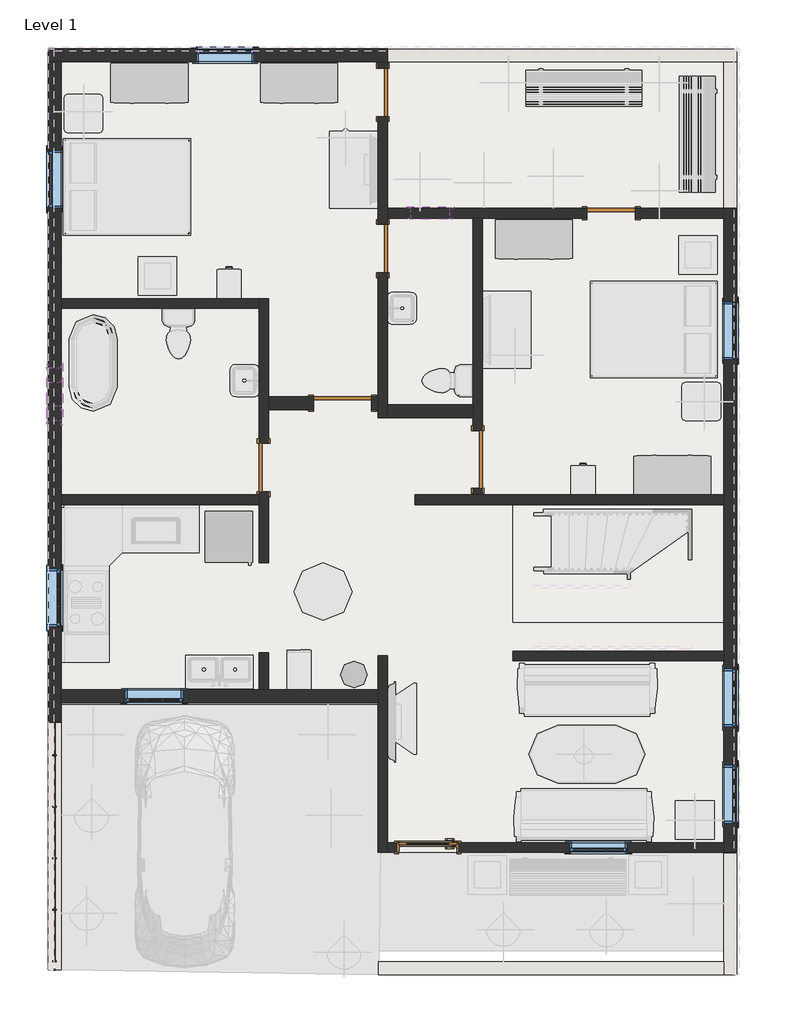
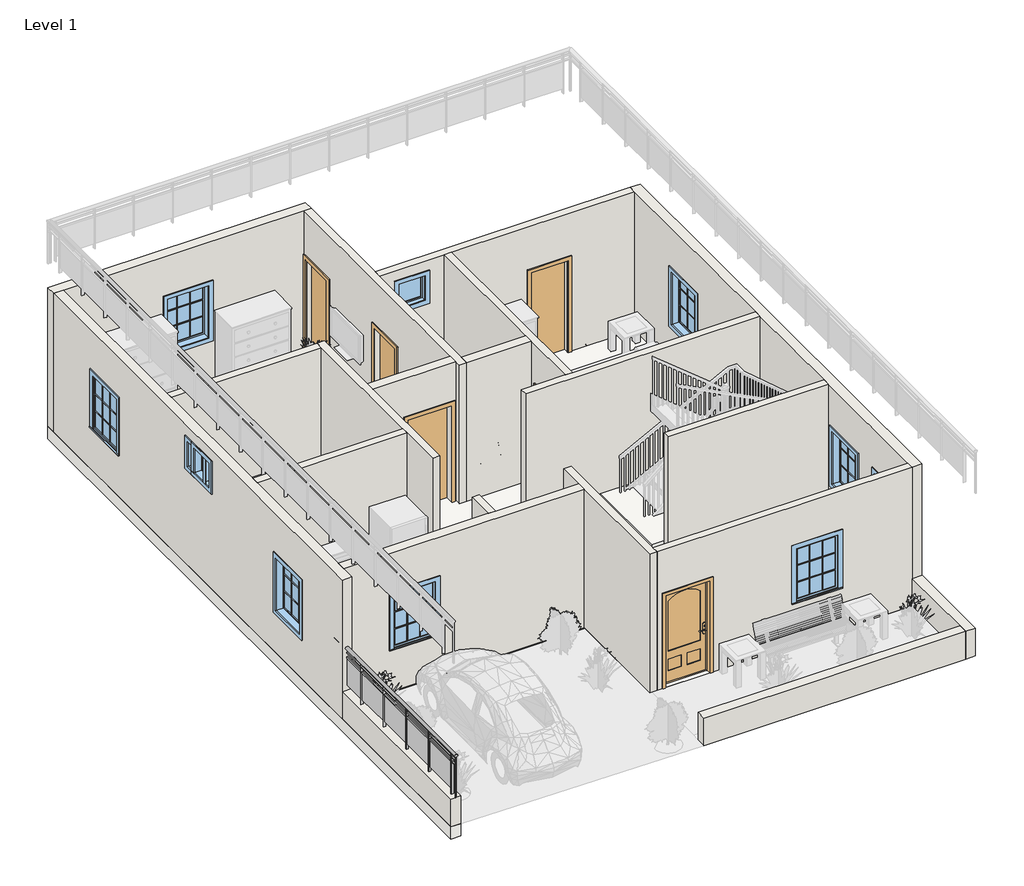
# One storey, part 1 of 4: 22 walls, 11 windows, 7 doors, 1 railing, 1 roof, 1 slab.
"""IFC4 building model written with IfcOpenShell, lengths in millimetres."""

from ifc_helpers import new_model, si_unit, point, frame, origin, origin_with_axes, place, context, project, spatial, polyline, ellipse_curve, trimmed, outline, extrude, faceted_brep, transform, mapped, element, save
from ifc_brep_helpers import plane_surface, extruded_surface, advanced_brep
from components import door_808aeb8e, door_255cab33, door_54dd4da4, door_16372e1c, window_29c06734, window_ce5e1bf6, window_5c190c7e, window_e41d21a6, window_3d781103

model = new_model("IFC4")

# Units and contexts
model_context = context("Model", 3, world=origin())
ifc_project = project(units=[si_unit("LENGTHUNIT", "METRE", prefix="MILLI")], contexts=[model_context])

# Site, building, storey
site = spatial("IfcSite", under=ifc_project)
building = spatial("IfcBuilding", under=site)
storey = spatial("IfcBuildingStorey", under=building, Name="Level 1", Elevation=0.0)

# Doors
placement = place(None, origin())
door_shape = door_808aeb8e(model_context)
element("IfcDoor", 1, ObjectType="36\" x 80\"", at=placement, inside=storey, context=model_context, shape_type="MappedRepresentation", body=[
    mapped(door_shape, transform((-6988.7866955, 3103.4537933, 0.0), x_axis=(1.0, 0.0, 0.0), y_axis=(0.0, 1.0, 0.0), z_axis=(0.0, 0.0, 1.0))),
])
door_2_shape = door_255cab33(model_context)
element("IfcDoor", 2, ObjectType="Single-Flush : 30\" x 80\"", at=placement, inside=storey, context=model_context, shape_type="MappedRepresentation", body=[
    mapped(door_2_shape, transform((-9579.5866955, 9094.6787933, 0.0), x_axis=(0.0, -1.0, 0.0), y_axis=(1.0, 0.0, 0.0), z_axis=(0.0, 0.0, 1.0))),
])
element("IfcDoor", 3, ObjectType="Single-Flush : 30\" x 80\"", at=placement, inside=storey, context=model_context, shape_type="MappedRepresentation", body=[
    mapped(door_2_shape, transform((-7699.9866955, 12549.0787933, 0.0), x_axis=(0.0, 1.0, 0.0), y_axis=(-1.0, 0.0, 0.0), z_axis=(0.0, 0.0, 1.0))),
])
element("IfcDoor", 4, ObjectType="Single-Flush : 30\" x 80\"", at=placement, inside=storey, context=model_context, shape_type="MappedRepresentation", body=[
    mapped(door_2_shape, transform((-7699.9866955, 15012.8787933, 0.0), x_axis=(0.0, 1.0, 0.0), y_axis=(-1.0, 0.0, 0.0), z_axis=(0.0, 0.0, 1.0))),
])
element("IfcDoor", 5, ObjectType="Single-Flush : 30\" x 80\"", at=placement, inside=storey, context=model_context, shape_type="MappedRepresentation", body=[
    mapped(door_2_shape, transform((-4093.1866955, 13107.8787933, 0.0), x_axis=(-1.0, 0.0, 0.0), y_axis=(0.0, -1.0, 0.0), z_axis=(0.0, 0.0, 1.0))),
])
door_3_shape = door_54dd4da4(model_context)
element("IfcDoor", 6, ObjectType="Single-Flush : 36\" x 84\"", at=placement, inside=storey, context=model_context, shape_type="MappedRepresentation", body=[
    mapped(door_3_shape, transform((-8334.9866955, 10110.6787933, 0.0), x_axis=(1.0, 0.0, 0.0), y_axis=(0.0, 1.0, 0.0), z_axis=(0.0, 0.0, 1.0))),
])
door_4_shape = door_16372e1c(model_context)
element("IfcDoor", 7, ObjectType="Single-Flush : 36\" x 84\"", at=placement, inside=storey, context=model_context, shape_type="MappedRepresentation", body=[
    mapped(door_4_shape, transform((-6201.3866955, 9221.6787933, 0.0), x_axis=(0.0, -1.0, 0.0), y_axis=(1.0, 0.0, 0.0), z_axis=(0.0, 0.0, 1.0))),
])

# Railing
element("IfcRailing", 8, ObjectType="Glass Panel - Bottom Fill", at=placement, inside=storey, context=model_context, shape_type="SolidModel", body=[
    advanced_brep(
    [(-12843.4866955, 5500.5787933, 1524.0), (-12919.6866955, 5500.5787933, 1524.0), (-12843.4866955, 1169.8787933, 1524.0), (-12919.6866955, 1169.8787933, 1524.0)],
    [
        (0, 1, ellipse_curve(frame((-12881.5866955, 5500.5787933, 1524.0), z_axis=(0.0, 1.0, 0.0), x_axis=(-1.0, 0.0, 0.0)), 38.1, 28.575)),
        (1, 0, ellipse_curve(frame((-12881.5866955, 5500.5787933, 1524.0), z_axis=(0.0, 1.0, 0.0), x_axis=(-1.0, 0.0, 0.0)), 38.1, 28.575)),
        (2, 3, ellipse_curve(frame((-12881.5866955, 1169.8787933, 1524.0), z_axis=(0.0, -1.0, 0.0), x_axis=(-1.0, 0.0, 0.0)), 38.1, 28.575)),
        (3, 2, ellipse_curve(frame((-12881.5866955, 1169.8787933, 1524.0), z_axis=(0.0, -1.0, 0.0), x_axis=(-1.0, 0.0, 0.0)), 38.1, 28.575)),
        (0, 2),
        (3, 1),
    ],
    [
        plane_surface(frame((-12881.5866955, 5500.5787933, 1524.0), z_axis=(0.0, 1.0, 0.0), x_axis=(0.0, 0.0, -1.0))),
        plane_surface(frame((-12881.5866955, 1169.8787933, 1524.0), z_axis=(0.0, -1.0, 0.0), x_axis=(0.0, 0.0, -1.0))),
        extruded_surface(trimmed(ellipse_curve(frame((-12881.5866955, 1169.8787933, 1524.0), z_axis=(0.0, 1.0, 0.0), x_axis=(-1.0, 0.0, 0.0)), 38.1, 28.575), [point((-12843.4866955, 1169.8787933, 1524.0))], [point((-12919.6866955, 1169.8787933, 1524.0))], True, "CARTESIAN"), (0.0, 4330.7, 0.0), 4330.7),
        extruded_surface(trimmed(ellipse_curve(frame((-12881.5866955, 1169.8787933, 1524.0), z_axis=(0.0, 1.0, 0.0), x_axis=(-1.0, 0.0, 0.0)), 38.1, 28.575), [point((-12919.6866955, 1169.8787933, 1524.0))], [point((-12843.4866955, 1169.8787933, 1524.0))], True, "CARTESIAN"), (0.0, 4330.7, 0.0), 4330.7),
    ],
    [
        (0, [[1, 2]]),
        (1, [[3, 4]]),
        (2, [[-1, 5, -4, 6]]),
        (3, [[-2, -6, -3, -5]]),
    ],
),
    extrude(outline(polyline([(-12894.2866955, 5500.5787933), (-12868.8866955, 5500.5787933), (-12868.8866955, 1169.8787933), (-12894.2866955, 1169.8787933), (-12894.2866955, 5500.5787933)])), frame((0.0, 0.0, 1409.7), z_axis=(0.0, 0.0, 1.0), x_axis=(1.0, 0.0, 0.0)), (0.0, 0.0, 1.0), 25.4),
    extrude(outline(polyline([(-12894.2866955, 5500.5787933), (-12868.8866955, 5500.5787933), (-12868.8866955, 1169.8787933), (-12894.2866955, 1169.8787933), (-12894.2866955, 5500.5787933)])), frame((0.0, 0.0, 1308.1), z_axis=(0.0, 0.0, 1.0), x_axis=(1.0, 0.0, 0.0)), (0.0, 0.0, 1.0), 25.4),
    extrude(outline(polyline([(-12906.9866955, 1309.5787933), (-12856.1866955, 1309.5787933), (-12856.1866955, 1296.8787933), (-12906.9866955, 1296.8787933), (-12906.9866955, 1309.5787933)])), frame((0.0, 0.0, 609.6), z_axis=(0.0, 0.0, 1.0), x_axis=(1.0, 0.0, 0.0)), (0.0, 0.0, 1.0), 885.6788223),
    extrude(outline(polyline([(-12875.0515385, 2116.0287933), (-12875.0515385, 1303.2287933), (-12881.4015385, 1303.2287933), (-12881.4015385, 2116.0287933), (-12875.0515385, 2116.0287933)])), frame((0.0, 0.0, 711.2), z_axis=(0.0, 0.0, 1.0), x_axis=(1.0, 0.0, 0.0)), (0.0, 0.0, 1.0), 596.9),
    extrude(outline(polyline([(-12906.9866955, 2122.3787933), (-12856.1866955, 2122.3787933), (-12856.1866955, 2109.6787933), (-12906.9866955, 2109.6787933), (-12906.9866955, 2122.3787933)])), frame((0.0, 0.0, 609.6), z_axis=(0.0, 0.0, 1.0), x_axis=(1.0, 0.0, 0.0)), (0.0, 0.0, 1.0), 885.6788223),
    extrude(outline(polyline([(-12875.0515385, 2928.8287933), (-12875.0515385, 2116.0287933), (-12881.4015385, 2116.0287933), (-12881.4015385, 2928.8287933), (-12875.0515385, 2928.8287933)])), frame((0.0, 0.0, 711.2), z_axis=(0.0, 0.0, 1.0), x_axis=(1.0, 0.0, 0.0)), (0.0, 0.0, 1.0), 596.9),
    extrude(outline(polyline([(-12906.9866955, 2935.1787933), (-12856.1866955, 2935.1787933), (-12856.1866955, 2922.4787933), (-12906.9866955, 2922.4787933), (-12906.9866955, 2935.1787933)])), frame((0.0, 0.0, 609.6), z_axis=(0.0, 0.0, 1.0), x_axis=(1.0, 0.0, 0.0)), (0.0, 0.0, 1.0), 885.6788223),
    extrude(outline(polyline([(-12875.0515385, 3741.6287933), (-12875.0515385, 2928.8287933), (-12881.4015385, 2928.8287933), (-12881.4015385, 3741.6287933), (-12875.0515385, 3741.6287933)])), frame((0.0, 0.0, 711.2), z_axis=(0.0, 0.0, 1.0), x_axis=(1.0, 0.0, 0.0)), (0.0, 0.0, 1.0), 596.9),
    extrude(outline(polyline([(-12906.9866955, 3747.9787933), (-12856.1866955, 3747.9787933), (-12856.1866955, 3735.2787933), (-12906.9866955, 3735.2787933), (-12906.9866955, 3747.9787933)])), frame((0.0, 0.0, 609.6), z_axis=(0.0, 0.0, 1.0), x_axis=(1.0, 0.0, 0.0)), (0.0, 0.0, 1.0), 885.6788223),
    extrude(outline(polyline([(-12875.0515385, 4554.4287933), (-12875.0515385, 3741.6287933), (-12881.4015385, 3741.6287933), (-12881.4015385, 4554.4287933), (-12875.0515385, 4554.4287933)])), frame((0.0, 0.0, 711.2), z_axis=(0.0, 0.0, 1.0), x_axis=(1.0, 0.0, 0.0)), (0.0, 0.0, 1.0), 596.9),
    extrude(outline(polyline([(-12906.9866955, 4560.7787933), (-12856.1866955, 4560.7787933), (-12856.1866955, 4548.0787933), (-12906.9866955, 4548.0787933), (-12906.9866955, 4560.7787933)])), frame((0.0, 0.0, 609.6), z_axis=(0.0, 0.0, 1.0), x_axis=(1.0, 0.0, 0.0)), (0.0, 0.0, 1.0), 885.6788223),
    extrude(outline(polyline([(-12875.0515385, 5367.2287933), (-12875.0515385, 4554.4287933), (-12881.4015385, 4554.4287933), (-12881.4015385, 5367.2287933), (-12875.0515385, 5367.2287933)])), frame((0.0, 0.0, 711.2), z_axis=(0.0, 0.0, 1.0), x_axis=(1.0, 0.0, 0.0)), (0.0, 0.0, 1.0), 596.9),
    extrude(outline(polyline([(-12906.9866955, 5373.5787933), (-12856.1866955, 5373.5787933), (-12856.1866955, 5360.8787933), (-12906.9866955, 5360.8787933), (-12906.9866955, 5373.5787933)])), frame((0.0, 0.0, 609.6), z_axis=(0.0, 0.0, 1.0), x_axis=(1.0, 0.0, 0.0)), (0.0, 0.0, 1.0), 885.6788223),
    extrude(outline(polyline([(-12891.1116955, 1182.5787933), (-12872.0616955, 1182.5787933), (-12872.0616955, 1163.5287933), (-12891.1116955, 1163.5287933), (-12891.1116955, 1182.5787933)])), frame((0.0, 0.0, 609.6), z_axis=(0.0, 0.0, 1.0), x_axis=(1.0, 0.0, 0.0)), (0.0, 0.0, 1.0), 885.6788223),
    extrude(outline(polyline([(-12891.1116955, 5506.9287933), (-12872.0616955, 5506.9287933), (-12872.0616955, 5487.8787933), (-12891.1116955, 5487.8787933), (-12891.1116955, 5506.9287933)])), frame((0.0, 0.0, 609.6), z_axis=(0.0, 0.0, 1.0), x_axis=(1.0, 0.0, 0.0)), (0.0, 0.0, 1.0), 885.6788223),
])

# Roof
element("IfcRoof", 9, ObjectType="Generic - 12\"", at=placement, inside=storey, context=model_context, shape_type="SweptSolid", body=[
    extrude(outline(polyline([(-5642.5866955, 8510.4787933), (-2111.9866955, 8510.4787933), (-2111.9866955, 6655.1793988), (-5642.5866955, 6655.1793988), (-5642.5866955, 8510.4787933)])), origin_with_axes(), (0.0, 0.0, 1.0), 304.8),
])

# Slab
element("IfcSlab", 10, ObjectType="Wood Joist 10\" - Wood Finish", at=placement, inside=storey, context=model_context, shape_type="SweptSolid", body=[
    extrude(outline(polyline([(-2111.9866955, 15698.6787933), (-2111.9866955, 3024.0787933), (-7776.1866955, 3024.0787933), (-7776.1866955, 5360.8787933), (-12754.5866955, 5360.8787933), (-12779.9866955, 5360.8787933), (-12779.9866955, 1169.8787933), (-12983.1866955, 1169.8787933), (-12983.1866955, 15698.6787933), (-2111.9866955, 15698.6787933)])), frame((0.0, 0.0, -273.05), z_axis=(0.0, 0.0, 1.0), x_axis=(1.0, 0.0, 0.0)), (0.0, 0.0, 1.0), 273.05),
])

# Walls
element("IfcWall", 11, ObjectType="Generic - 8\"", at=placement, inside=storey, context=model_context, shape_type="Brep", body=[
    faceted_brep([(-12983.1866955, 15495.4787933, 0.0), (-12779.9866955, 15495.4787933, 0.0), (-7776.1866955, 15495.4787933, 0.0), (-7699.9866955, 15495.4787933, 0.0), (-7699.9866955, 15495.4787933, 609.6), (-7623.7866955, 15495.4787933, 609.6), (-7623.7866955, 15495.4787933, 3048.0), (-7776.1866955, 15495.4787933, 3048.0), (-12779.9866955, 15495.4787933, 3048.0), (-12983.1866955, 15495.4787933, 3048.0), (-9731.9866955, 15495.4787933, 2133.6), (-9731.9866955, 15495.4787933, 914.4), (-10646.3866955, 15495.4787933, 914.4), (-10646.3866955, 15495.4787933, 2133.6), (-12983.1866955, 15698.6787933, 0.0), (-12983.1866955, 15698.6787933, 3048.0), (-7623.7866955, 15698.6787933, 3048.0), (-7623.7866955, 15698.6787933, 609.6), (-7699.9866955, 15698.6787933, 609.6), (-7699.9866955, 15698.6787933, 0.0), (-9731.9866955, 15698.6787933, 2133.6), (-10646.3866955, 15698.6787933, 2133.6), (-10646.3866955, 15698.6787933, 914.4), (-9731.9866955, 15698.6787933, 914.4)], [[[0, 1, 2, 3, 4, 5, 6, 7, 8, 9], [10, 11, 12, 13]], [[14, 15, 16, 17, 18, 19], [20, 21, 22, 23]], [[3, 2, 1, 0, 14, 19]], [[0, 9, 15, 14]], [[11, 10, 20, 23]], [[12, 11, 23, 22]], [[13, 12, 22, 21]], [[10, 13, 21, 20]], [[4, 3, 19, 18]], [[17, 5, 4, 18]], [[6, 5, 17, 16]], [[9, 8, 7, 6, 16, 15]]]),
])
element("IfcWall", 12, ObjectType="Generic - 8\"", at=placement, inside=storey, context=model_context, shape_type="Brep", body=[
    faceted_brep([(-2315.1866955, 15495.4787933, 0.0), (-2315.1866955, 13184.0787933, 0.0), (-2315.1866955, 13107.8787933, 0.0), (-2315.1866955, 13107.8787933, 609.6), (-2315.1866955, 13184.0787933, 609.6), (-2315.1866955, 15495.4787933, 609.6), (-2111.9866955, 15495.4787933, 0.0), (-2111.9866955, 15495.4787933, 609.6), (-2111.9866955, 13184.0787933, 609.6), (-2111.9866955, 13107.8787933, 609.6), (-2111.9866955, 13107.8787933, 0.0)], [[[0, 1, 2, 3, 4, 5]], [[6, 7, 8, 9, 10]], [[2, 1, 0, 6, 10]], [[3, 2, 10, 9]], [[5, 4, 3, 9, 8, 7]], [[0, 5, 7, 6]]]),
])
element("IfcWall", 13, ObjectType="Generic - 8\"", at=placement, inside=storey, context=model_context, shape_type="SweptSolid", body=[
    extrude(outline(polyline([(-7763.4866955, 1296.8787933), (-2315.1866955, 1296.8787933), (-2315.1866955, 1093.6787933), (-7763.4866955, 1093.6787933), (-7763.4866955, 1296.8787933)])), origin_with_axes(), (0.0, 0.0, 1.0), 609.6),
])
element("IfcWall", 14, ObjectType="Generic - 8\"", at=placement, inside=storey, context=model_context, shape_type="SweptSolid", body=[
    extrude(outline(polyline([(-12779.9866955, 5068.7787933), (-12779.9866955, 1169.8787933), (-12983.1866955, 1169.8787933), (-12983.1866955, 5068.7787933), (-12779.9866955, 5068.7787933)])), origin_with_axes(), (0.0, 0.0, 1.0), 609.6),
])
element("IfcWall", 15, ObjectType="Generic - 8\"", at=placement, inside=storey, context=model_context, shape_type="SweptSolid", body=[
    extrude(outline(polyline([(2133.6, -7877.7866955), (0.0, -7877.7866955), (0.0, -7776.1866955), (3048.0, -7776.1866955), (3048.0, -9503.3866955), (0.0, -9503.3866955), (0.0, -8792.1866955), (2133.6, -8792.1866955), (2133.6, -7877.7866955)])), frame((0.0, 10009.0787933, 0.0), z_axis=(0.0, 1.0, 0.0), x_axis=(0.0, 0.0, 1.0)), (0.0, 0.0, 1.0), 203.2),
])
element("IfcWall", 16, ObjectType="Generic - 8\"", at=placement, inside=storey, context=model_context, shape_type="SweptSolid", body=[
    extrude(outline(polyline([(-7623.7866955, 10085.2787933), (-6277.5866955, 10085.2787933), (-6277.5866955, 9882.0787933), (-7623.7866955, 9882.0787933), (-7623.7866955, 10085.2787933)])), origin_with_axes(), (0.0, 0.0, 1.0), 3048.0),
])
element("IfcWall", 17, ObjectType="Generic - 8\"", at=placement, inside=storey, context=model_context, shape_type="Brep", body=[
    faceted_brep([(-12779.9866955, 5386.2787933, 0.0), (-7776.1866955, 5386.2787933, 0.0), (-7776.1866955, 5386.2787933, 3048.0), (-12779.9866955, 5386.2787933, 3048.0), (-11763.9866955, 5386.2787933, 2133.6), (-10849.5866955, 5386.2787933, 2133.6), (-10849.5866955, 5386.2787933, 914.4), (-11763.9866955, 5386.2787933, 914.4), (-12779.9866955, 5589.4787933, 0.0), (-12779.9866955, 5589.4787933, 3048.0), (-9655.7866955, 5589.4787933, 3048.0), (-9503.3866955, 5589.4787933, 3048.0), (-7776.1866955, 5589.4787933, 3048.0), (-7776.1866955, 5589.4787933, 0.0), (-9503.3866955, 5589.4787933, 0.0), (-9655.7866955, 5589.4787933, 0.0), (-11763.9866955, 5589.4787933, 2133.6), (-11763.9866955, 5589.4787933, 914.4), (-10849.5866955, 5589.4787933, 914.4), (-10849.5866955, 5589.4787933, 2133.6)], [[[0, 1, 2, 3], [4, 5, 6, 7]], [[8, 9, 10, 11, 12, 13, 14, 15], [16, 17, 18, 19]], [[1, 0, 8, 15, 14, 13]], [[0, 3, 9, 8]], [[2, 1, 13, 12]], [[17, 16, 4, 7]], [[18, 17, 7, 6]], [[19, 18, 6, 5]], [[16, 19, 5, 4]], [[3, 2, 12, 11, 10, 9]]]),
])
element("IfcWall", 18, ObjectType="Generic - 8\"", at=placement, inside=storey, context=model_context, shape_type="Brep", body=[
    faceted_brep([(-2315.1866955, 3011.3787933, 0.0), (-2315.1866955, 1296.8787933, 0.0), (-2315.1866955, 1093.6787933, 0.0), (-2315.1866955, 1093.6787933, 609.6), (-2315.1866955, 1296.8787933, 609.6), (-2315.1866955, 3011.3787933, 609.6), (-2111.9866955, 3011.3787933, 0.0), (-2111.9866955, 3011.3787933, 609.6), (-2111.9866955, 1093.6787933, 609.6), (-2111.9866955, 1093.6787933, 0.0)], [[[0, 1, 2, 3, 4, 5]], [[6, 7, 8, 9]], [[2, 1, 0, 6, 9]], [[5, 4, 3, 8, 7]], [[0, 5, 7, 6]], [[3, 2, 9, 8]]]),
])
element("IfcWall", 19, ObjectType="Generic - 8\"", at=placement, inside=storey, context=model_context, shape_type="Brep", body=[
    faceted_brep([(-12779.9866955, 5094.1787933, 0.0), (-12779.9866955, 5386.2787933, 0.0), (-12779.9866955, 5589.4787933, 0.0), (-12779.9866955, 8510.4787933, 0.0), (-12779.9866955, 8662.8787933, 0.0), (-12779.9866955, 11609.2787933, 0.0), (-12779.9866955, 11761.6787933, 0.0), (-12779.9866955, 15495.4787933, 0.0), (-12779.9866955, 15495.4787933, 3048.0), (-12779.9866955, 11761.6787933, 3048.0), (-12779.9866955, 11609.2787933, 3048.0), (-12779.9866955, 8662.8787933, 3048.0), (-12779.9866955, 8510.4787933, 3048.0), (-12779.9866955, 5589.4787933, 3048.0), (-12779.9866955, 5386.2787933, 3048.0), (-12779.9866955, 5094.1787933, 3048.0), (-12779.9866955, 14098.4787933, 2133.6), (-12779.9866955, 14098.4787933, 914.4), (-12779.9866955, 13184.0787933, 914.4), (-12779.9866955, 13184.0787933, 2133.6), (-12779.9866955, 7494.4787933, 2133.6), (-12779.9866955, 7494.4787933, 914.4), (-12779.9866955, 6580.0787933, 914.4), (-12779.9866955, 6580.0787933, 2133.6), (-12779.9866955, 10669.4787933, 2159.0), (-12779.9866955, 9831.2787933, 2159.0), (-12779.9866955, 9831.2787933, 2768.6), (-12779.9866955, 10669.4787933, 2768.6), (-12983.1866955, 15495.4787933, 0.0), (-12983.1866955, 5094.1787933, 0.0), (-12983.1866955, 5094.1787933, 3048.0), (-12983.1866955, 15495.4787933, 3048.0), (-12983.1866955, 14098.4787933, 2133.6), (-12983.1866955, 13184.0787933, 2133.6), (-12983.1866955, 13184.0787933, 914.4), (-12983.1866955, 14098.4787933, 914.4), (-12983.1866955, 7494.4787933, 2133.6), (-12983.1866955, 6580.0787933, 2133.6), (-12983.1866955, 6580.0787933, 914.4), (-12983.1866955, 7494.4787933, 914.4), (-12983.1866955, 10669.4787933, 2768.6), (-12983.1866955, 9831.2787933, 2768.6), (-12983.1866955, 9831.2787933, 2159.0), (-12983.1866955, 10669.4787933, 2159.0)], [[[0, 1, 2, 3, 4, 5, 6, 7, 8, 9, 10, 11, 12, 13, 14, 15], [16, 17, 18, 19], [20, 21, 22, 23], [24, 25, 26, 27]], [[28, 29, 30, 31], [32, 33, 34, 35], [36, 37, 38, 39], [40, 41, 42, 43]], [[7, 6, 5, 4, 3, 2, 1, 0, 29, 28]], [[0, 15, 30, 29]], [[8, 7, 28, 31]], [[17, 16, 32, 35]], [[18, 17, 35, 34]], [[19, 18, 34, 33]], [[16, 19, 33, 32]], [[21, 20, 36, 39]], [[22, 21, 39, 38]], [[23, 22, 38, 37]], [[20, 23, 37, 36]], [[42, 41, 26, 25]], [[42, 25, 24, 43]], [[26, 41, 40, 27]], [[43, 24, 27, 40]], [[15, 14, 13, 12, 11, 10, 9, 8, 31, 30]]]),
])
element("IfcWall", 20, ObjectType="Generic - 8\"", at=placement, inside=storey, context=model_context, shape_type="Brep", body=[
    faceted_brep([(-7699.9866955, 15495.4787933, 0.0), (-7623.7866955, 15495.4787933, 0.0), (-2315.1866955, 15495.4787933, 0.0), (-2111.9866955, 15495.4787933, 0.0), (-2111.9866955, 15495.4787933, 609.6), (-2315.1866955, 15495.4787933, 609.6), (-7623.7866955, 15495.4787933, 609.6), (-7699.9866955, 15495.4787933, 609.6), (-7699.9866955, 15698.6787933, 0.0), (-7699.9866955, 15698.6787933, 609.6), (-7623.7866955, 15698.6787933, 609.6), (-2111.9866955, 15698.6787933, 609.6), (-2111.9866955, 15698.6787933, 0.0)], [[[0, 1, 2, 3, 4, 5, 6, 7]], [[8, 9, 10, 11, 12]], [[3, 2, 1, 0, 8, 12]], [[7, 6, 5, 4, 11, 10, 9]], [[0, 7, 9, 8]], [[4, 3, 12, 11]]]),
])
element("IfcWall", 21, ObjectType="Generic - 8\"", at=placement, inside=storey, context=model_context, shape_type="Brep", body=[
    faceted_brep([(-2315.1866955, 13107.8787933, 0.0), (-2315.1866955, 13031.6787933, 0.0), (-2315.1866955, 8662.8787933, 0.0), (-2315.1866955, 8510.4787933, 0.0), (-2315.1866955, 6199.0787933, 0.0), (-2315.1866955, 6046.6787933, 0.0), (-2315.1866955, 3176.4787933, 0.0), (-2315.1866955, 3036.7787933, 0.0), (-2315.1866955, 3036.7787933, 3048.0), (-2315.1866955, 3176.4787933, 3048.0), (-2315.1866955, 6046.6787933, 3048.0), (-2315.1866955, 6199.0787933, 3048.0), (-2315.1866955, 8510.4787933, 3048.0), (-2315.1866955, 8662.8787933, 3048.0), (-2315.1866955, 13031.6787933, 3048.0), (-2315.1866955, 13184.0787933, 3048.0), (-2315.1866955, 13184.0787933, 609.6), (-2315.1866955, 13107.8787933, 609.6), (-2315.1866955, 10796.4787933, 2133.6), (-2315.1866955, 10796.4787933, 914.4), (-2315.1866955, 11710.8787933, 914.4), (-2315.1866955, 11710.8787933, 2133.6), (-2315.1866955, 3481.2787933, 2133.6), (-2315.1866955, 3481.2787933, 914.4), (-2315.1866955, 4395.6787933, 914.4), (-2315.1866955, 4395.6787933, 2133.6), (-2315.1866955, 5005.2787933, 2133.6), (-2315.1866955, 5005.2787933, 914.4), (-2315.1866955, 5919.6787933, 914.4), (-2315.1866955, 5919.6787933, 2133.6), (-2111.9866955, 13107.8787933, 0.0), (-2111.9866955, 13107.8787933, 609.6), (-2111.9866955, 13184.0787933, 609.6), (-2111.9866955, 13184.0787933, 3048.0), (-2111.9866955, 3036.7787933, 3048.0), (-2111.9866955, 3036.7787933, 0.0), (-2111.9866955, 10796.4787933, 2133.6), (-2111.9866955, 11710.8787933, 2133.6), (-2111.9866955, 11710.8787933, 914.4), (-2111.9866955, 10796.4787933, 914.4), (-2111.9866955, 3481.2787933, 2133.6), (-2111.9866955, 4395.6787933, 2133.6), (-2111.9866955, 4395.6787933, 914.4), (-2111.9866955, 3481.2787933, 914.4), (-2111.9866955, 5005.2787933, 2133.6), (-2111.9866955, 5919.6787933, 2133.6), (-2111.9866955, 5919.6787933, 914.4), (-2111.9866955, 5005.2787933, 914.4)], [[[0, 1, 2, 3, 4, 5, 6, 7, 8, 9, 10, 11, 12, 13, 14, 15, 16, 17], [18, 19, 20, 21], [22, 23, 24, 25], [26, 27, 28, 29]], [[30, 31, 32, 33, 34, 35], [36, 37, 38, 39], [40, 41, 42, 43], [44, 45, 46, 47]], [[7, 6, 5, 4, 3, 2, 1, 0, 30, 35]], [[8, 7, 35, 34]], [[18, 21, 37, 36]], [[21, 20, 38, 37]], [[20, 19, 39, 38]], [[19, 18, 36, 39]], [[22, 25, 41, 40]], [[25, 24, 42, 41]], [[24, 23, 43, 42]], [[23, 22, 40, 43]], [[26, 29, 45, 44]], [[29, 28, 46, 45]], [[28, 27, 47, 46]], [[27, 26, 44, 47]], [[0, 17, 31, 30]], [[16, 32, 31, 17]], [[16, 15, 33, 32]], [[15, 14, 13, 12, 11, 10, 9, 8, 34, 33]]]),
])
element("IfcWall", 22, ObjectType="INNER 6\"", at=placement, inside=storey, context=model_context, shape_type="Brep", body=[
    faceted_brep([(-7776.1866955, 15495.4787933, 0.0), (-7776.1866955, 15393.8787933, 0.0), (-7776.1866955, 15393.8787933, 2032.0), (-7776.1866955, 14631.8787933, 2032.0), (-7776.1866955, 14631.8787933, 0.0), (-7776.1866955, 12930.0787933, 0.0), (-7776.1866955, 12930.0787933, 2032.0), (-7776.1866955, 12168.0787933, 2032.0), (-7776.1866955, 12168.0787933, 0.0), (-7776.1866955, 10212.2787933, 0.0), (-7776.1866955, 10009.0787933, 0.0), (-7776.1866955, 9882.0787933, 0.0), (-7776.1866955, 9882.0787933, 3048.0), (-7776.1866955, 10009.0787933, 3048.0), (-7776.1866955, 10212.2787933, 3048.0), (-7776.1866955, 15495.4787933, 3048.0), (-7623.7866955, 15393.8787933, 2032.0), (-7623.7866955, 15393.8787933, 0.0), (-7623.7866955, 15495.4787933, 0.0), (-7623.7866955, 15495.4787933, 609.6), (-7623.7866955, 15495.4787933, 3048.0), (-7623.7866955, 13184.0787933, 3048.0), (-7623.7866955, 13031.6787933, 3048.0), (-7623.7866955, 10085.2787933, 3048.0), (-7623.7866955, 9882.0787933, 3048.0), (-7623.7866955, 9882.0787933, 0.0), (-7623.7866955, 10085.2787933, 0.0), (-7623.7866955, 12168.0787933, 0.0), (-7623.7866955, 12168.0787933, 2032.0), (-7623.7866955, 12930.0787933, 2032.0), (-7623.7866955, 12930.0787933, 0.0), (-7623.7866955, 13031.6787933, 0.0), (-7623.7866955, 13184.0787933, 0.0), (-7623.7866955, 14631.8787933, 0.0), (-7623.7866955, 14631.8787933, 2032.0), (-7699.9866955, 15495.4787933, 0.0)], [[[0, 1, 2, 3, 4, 5, 6, 7, 8, 9, 10, 11, 12, 13, 14, 15]], [[16, 17, 18, 19, 20, 21, 22, 23, 24, 25, 26, 27, 28, 29, 30, 31, 32, 33, 34]], [[27, 26, 25, 11, 10, 9, 8]], [[18, 17, 1, 0, 35]], [[33, 32, 31, 30, 5, 4]], [[12, 11, 25, 24]], [[6, 5, 30, 29]], [[7, 6, 29, 28]], [[8, 7, 28, 27]], [[2, 1, 17, 16]], [[3, 2, 16, 34]], [[4, 3, 34, 33]], [[15, 20, 19, 18, 35, 0]], [[15, 14, 13, 12, 24, 23, 22, 21, 20]]]),
])
element("IfcWall", 23, ObjectType="INNER 6\"", at=placement, inside=storey, context=model_context, shape_type="SweptSolid", body=[
    extrude(outline(polyline([(-9503.3866955, 6173.6787933), (-9503.3866955, 5589.4787933), (-9655.7866955, 5589.4787933), (-9655.7866955, 6173.6787933), (-9503.3866955, 6173.6787933)])), origin_with_axes(), (0.0, 0.0, 1.0), 3048.0),
])
element("IfcWall", 24, ObjectType="INNER 6\"", at=placement, inside=storey, context=model_context, shape_type="SweptSolid", body=[
    extrude(outline(polyline([(-12779.9866955, 11761.6787933), (-9655.7866955, 11761.6787933), (-9655.7866955, 11609.2787933), (-12779.9866955, 11609.2787933), (-12779.9866955, 11761.6787933)])), origin_with_axes(), (0.0, 0.0, 1.0), 3048.0),
])
element("IfcWall", 25, ObjectType="INNER 6\"", at=placement, inside=storey, context=model_context, shape_type="SweptSolid", body=[
    extrude(outline(polyline([(-9655.7866955, 8510.4787933), (-12779.9866955, 8510.4787933), (-12779.9866955, 8662.8787933), (-9655.7866955, 8662.8787933), (-9655.7866955, 8510.4787933)])), origin_with_axes(), (0.0, 0.0, 1.0), 3048.0),
])
element("IfcWall", 26, ObjectType="INNER 6\"", at=placement, inside=storey, context=model_context, shape_type="Brep", body=[
    faceted_brep([(-7191.9866955, 8510.4787933, 0.0), (-2315.1866955, 8510.4787933, 0.0), (-2315.1866955, 8510.4787933, 3048.0), (-7191.9866955, 8510.4787933, 3048.0), (-7191.9866955, 8662.8787933, 0.0), (-7191.9866955, 8662.8787933, 3048.0), (-6277.5866955, 8662.8787933, 3048.0), (-6125.1866955, 8662.8787933, 3048.0), (-2315.1866955, 8662.8787933, 3048.0), (-2315.1866955, 8662.8787933, 0.0), (-6125.1866955, 8662.8787933, 0.0), (-6277.5866955, 8662.8787933, 0.0)], [[[0, 1, 2, 3]], [[4, 5, 6, 7, 8, 9, 10, 11]], [[1, 0, 4, 11, 10, 9]], [[0, 3, 5, 4]], [[2, 1, 9, 8]], [[3, 2, 8, 7, 6, 5]]]),
])
element("IfcWall", 27, ObjectType="INNER 6\"", at=placement, inside=storey, context=model_context, shape_type="Brep", body=[
    faceted_brep([(-7623.7866955, 13031.6787933, 0.0), (-6277.5866955, 13031.6787933, 0.0), (-6125.1866955, 13031.6787933, 0.0), (-4474.1866955, 13031.6787933, 0.0), (-4474.1866955, 13031.6787933, 2032.0), (-3712.1866955, 13031.6787933, 2032.0), (-3712.1866955, 13031.6787933, 0.0), (-2315.1866955, 13031.6787933, 0.0), (-2315.1866955, 13031.6787933, 3048.0), (-6125.1866955, 13031.6787933, 3048.0), (-6277.5866955, 13031.6787933, 3048.0), (-7623.7866955, 13031.6787933, 3048.0), (-6645.8866955, 13031.6787933, 2768.6), (-6645.8866955, 13031.6787933, 2159.0), (-7255.4866955, 13031.6787933, 2159.0), (-7255.4866955, 13031.6787933, 2768.6), (-4474.1866955, 13184.0787933, 2032.0), (-4474.1866955, 13184.0787933, 0.0), (-7623.7866955, 13184.0787933, 0.0), (-7623.7866955, 13184.0787933, 3048.0), (-2315.1866955, 13184.0787933, 3048.0), (-2315.1866955, 13184.0787933, 609.6), (-2315.1866955, 13184.0787933, 0.0), (-3712.1866955, 13184.0787933, 0.0), (-3712.1866955, 13184.0787933, 2032.0), (-6645.8866955, 13184.0787933, 2768.6), (-7255.4866955, 13184.0787933, 2768.6), (-7255.4866955, 13184.0787933, 2159.0), (-6645.8866955, 13184.0787933, 2159.0), (-2315.1866955, 13107.8787933, 0.0)], [[[0, 1, 2, 3, 4, 5, 6, 7, 8, 9, 10, 11], [12, 13, 14, 15]], [[16, 17, 18, 19, 20, 21, 22, 23, 24], [25, 26, 27, 28]], [[23, 22, 29, 7, 6]], [[18, 17, 3, 2, 1, 0]], [[0, 11, 19, 18]], [[4, 3, 17, 16]], [[5, 4, 16, 24]], [[6, 5, 24, 23]], [[13, 12, 25, 28]], [[14, 13, 28, 27]], [[15, 14, 27, 26]], [[12, 15, 26, 25]], [[7, 29, 22, 21, 20, 8]], [[11, 10, 9, 8, 20, 19]]]),
])
element("IfcWall", 28, ObjectType="INNER 6\"", at=placement, inside=storey, context=model_context, shape_type="Brep", body=[
    faceted_brep([(-6277.5866955, 8764.4787933, 2133.6), (-6277.5866955, 8764.4787933, 0.0), (-6277.5866955, 8662.8787933, 0.0), (-6277.5866955, 8662.8787933, 3048.0), (-6277.5866955, 9882.0787933, 3048.0), (-6277.5866955, 10085.2787933, 3048.0), (-6277.5866955, 13031.6787933, 3048.0), (-6277.5866955, 13031.6787933, 0.0), (-6277.5866955, 10085.2787933, 0.0), (-6277.5866955, 9882.0787933, 0.0), (-6277.5866955, 9678.8787933, 0.0), (-6277.5866955, 9678.8787933, 2133.6), (-6125.1866955, 8662.8787933, 0.0), (-6125.1866955, 8764.4787933, 0.0), (-6125.1866955, 8764.4787933, 2133.6), (-6125.1866955, 9678.8787933, 2133.6), (-6125.1866955, 9678.8787933, 0.0), (-6125.1866955, 13031.6787933, 0.0), (-6125.1866955, 13031.6787933, 3048.0), (-6125.1866955, 8662.8787933, 3048.0)], [[[0, 1, 2, 3, 4, 5, 6, 7, 8, 9, 10, 11]], [[12, 13, 14, 15, 16, 17, 18, 19]], [[2, 1, 13, 12]], [[10, 9, 8, 7, 17, 16]], [[7, 6, 18, 17]], [[3, 2, 12, 19]], [[14, 13, 1, 0]], [[15, 14, 0, 11]], [[16, 15, 11, 10]], [[6, 5, 4, 3, 19, 18]]]),
])
element("IfcWall", 29, ObjectType="INNER 6\"", at=placement, inside=storey, context=model_context, shape_type="Brep", body=[
    faceted_brep([(-7623.7866955, 3024.0787933, 0.0), (-7623.7866955, 3176.4787933, 0.0), (-7623.7866955, 6122.8787933, 0.0), (-7623.7866955, 6122.8787933, 3048.0), (-7623.7866955, 3176.4787933, 3048.0), (-7623.7866955, 3024.0787933, 3048.0), (-7776.1866955, 3024.0787933, 0.0), (-7776.1866955, 3024.0787933, 3048.0), (-7776.1866955, 5386.2787933, 3048.0), (-7776.1866955, 5589.4787933, 3048.0), (-7776.1866955, 6122.8787933, 3048.0), (-7776.1866955, 6122.8787933, 0.0), (-7776.1866955, 5589.4787933, 0.0), (-7776.1866955, 5386.2787933, 0.0)], [[[0, 1, 2, 3, 4, 5]], [[6, 7, 8, 9, 10, 11, 12, 13]], [[2, 1, 0, 6, 13, 12, 11]], [[3, 2, 11, 10]], [[0, 5, 7, 6]], [[5, 4, 3, 10, 9, 8, 7]]]),
])
element("IfcWall", 30, ObjectType="INNER 6\"", at=placement, inside=storey, context=model_context, shape_type="Brep", body=[
    faceted_brep([(-7623.7866955, 3176.4787933, 0.0), (-7623.7866955, 3176.4787933, 3048.0), (-2315.1866955, 3176.4787933, 3048.0), (-2315.1866955, 3176.4787933, 0.0), (-6506.1866955, 3176.4787933, 0.0), (-6506.1866955, 3176.4787933, 2057.4), (-7471.3866955, 3176.4787933, 2057.4), (-7471.3866955, 3176.4787933, 0.0), (-4753.5866955, 3176.4787933, 2133.6), (-4753.5866955, 3176.4787933, 914.4), (-3839.1866955, 3176.4787933, 914.4), (-3839.1866955, 3176.4787933, 2133.6), (-7623.7866955, 3024.0787933, 3048.0), (-7623.7866955, 3024.0787933, 0.0), (-7471.3866955, 3024.0787933, 0.0), (-7471.3866955, 3024.0787933, 2057.4), (-6506.1866955, 3024.0787933, 2057.4), (-6506.1866955, 3024.0787933, 0.0), (-2315.1866955, 3024.0787933, 0.0), (-2315.1866955, 3024.0787933, 3048.0), (-4753.5866955, 3024.0787933, 2133.6), (-3839.1866955, 3024.0787933, 2133.6), (-3839.1866955, 3024.0787933, 914.4), (-4753.5866955, 3024.0787933, 914.4), (-2315.1866955, 3036.7787933, 0.0), (-2315.1866955, 3036.7787933, 3048.0)], [[[0, 1, 2, 3, 4, 5, 6, 7], [8, 9, 10, 11]], [[12, 13, 14, 15, 16, 17, 18, 19], [20, 21, 22, 23]], [[13, 0, 7, 14]], [[3, 24, 18, 17, 4]], [[1, 0, 13, 12]], [[16, 5, 4, 17]], [[5, 16, 15, 6]], [[6, 15, 14, 7]], [[3, 2, 25, 19, 18, 24]], [[9, 8, 20, 23]], [[10, 9, 23, 22]], [[11, 10, 22, 21]], [[8, 11, 21, 20]], [[2, 1, 12, 19, 25]]]),
])
element("IfcWall", 31, ObjectType="INNER 6\"", at=placement, inside=storey, context=model_context, shape_type="Brep", body=[
    faceted_brep([(-9503.3866955, 7596.0787933, 0.0), (-9503.3866955, 8713.6787933, 0.0), (-9503.3866955, 8713.6787933, 2032.0), (-9503.3866955, 9475.6787933, 2032.0), (-9503.3866955, 9475.6787933, 0.0), (-9503.3866955, 10009.0787933, 0.0), (-9503.3866955, 10212.2787933, 0.0), (-9503.3866955, 11761.6787933, 0.0), (-9503.3866955, 11761.6787933, 3048.0), (-9503.3866955, 10212.2787933, 3048.0), (-9503.3866955, 10009.0787933, 3048.0), (-9503.3866955, 7596.0787933, 3048.0), (-9655.7866955, 8713.6787933, 2032.0), (-9655.7866955, 8713.6787933, 0.0), (-9655.7866955, 8662.8787933, 0.0), (-9655.7866955, 8510.4787933, 0.0), (-9655.7866955, 7596.0787933, 0.0), (-9655.7866955, 7596.0787933, 3048.0), (-9655.7866955, 8510.4787933, 3048.0), (-9655.7866955, 8662.8787933, 3048.0), (-9655.7866955, 11609.2787933, 3048.0), (-9655.7866955, 11761.6787933, 3048.0), (-9655.7866955, 11761.6787933, 0.0), (-9655.7866955, 11609.2787933, 0.0), (-9655.7866955, 9475.6787933, 0.0), (-9655.7866955, 9475.6787933, 2032.0)], [[[0, 1, 2, 3, 4, 5, 6, 7, 8, 9, 10, 11]], [[12, 13, 14, 15, 16, 17, 18, 19, 20, 21, 22, 23, 24, 25]], [[24, 23, 22, 7, 6, 5, 4]], [[16, 15, 14, 13, 1, 0]], [[0, 11, 17, 16]], [[8, 7, 22, 21]], [[4, 3, 25, 24]], [[3, 2, 12, 25]], [[2, 1, 13, 12]], [[11, 10, 9, 8, 21, 20, 19, 18, 17]]]),
])
element("IfcWall", 32, ObjectType="INNER 6\"", at=placement, inside=storey, context=model_context, shape_type="SweptSolid", body=[
    extrude(outline(polyline([(-5642.5866955, 6199.0787933), (-2315.1866955, 6199.0787933), (-2315.1866955, 6046.6787933), (-5642.5866955, 6046.6787933), (-5642.5866955, 6199.0787933)])), origin_with_axes(), (0.0, 0.0, 1.0), 3048.0),
])

# Windows
window_shape = window_29c06734(model_context)
element("IfcWindow", 33, ObjectType="Casement 3x3 with Trim : 36\" x 48\"", at=placement, inside=storey, context=model_context, shape_type="MappedRepresentation", body=[
    mapped(window_shape, transform((-12881.5866955, 13641.2787933, 0.0), x_axis=(0.0, 1.0, 0.0), y_axis=(-1.0, 0.0, 0.0), z_axis=(0.0, 0.0, 1.0))),
])
element("IfcWindow", 34, ObjectType="Casement 3x3 with Trim : 36\" x 48\"", at=placement, inside=storey, context=model_context, shape_type="MappedRepresentation", body=[
    mapped(window_shape, transform((-10189.1866955, 15597.0787933, 0.0), x_axis=(1.0, 0.0, 0.0), y_axis=(0.0, 1.0, 0.0), z_axis=(0.0, 0.0, 1.0))),
])
element("IfcWindow", 35, ObjectType="Casement 3x3 with Trim : 36\" x 48\"", at=placement, inside=storey, context=model_context, shape_type="MappedRepresentation", body=[
    mapped(window_shape, transform((-2213.5866955, 11253.6787933, 0.0), x_axis=(0.0, -1.0, 0.0), y_axis=(1.0, 0.0, 0.0), z_axis=(0.0, 0.0, 1.0))),
])
element("IfcWindow", 36, ObjectType="Casement 3x3 with Trim : 36\" x 48\"", at=placement, inside=storey, context=model_context, shape_type="MappedRepresentation", body=[
    mapped(window_shape, transform((-11306.7866955, 5487.8787933, 0.0), x_axis=(-1.0, 0.0, 0.0), y_axis=(0.0, -1.0, 0.0), z_axis=(0.0, 0.0, 1.0))),
])
element("IfcWindow", 37, ObjectType="Casement 3x3 with Trim : 36\" x 48\"", at=placement, inside=storey, context=model_context, shape_type="MappedRepresentation", body=[
    mapped(window_shape, transform((-2213.5866955, 3938.4787933, 0.0), x_axis=(0.0, -1.0, 0.0), y_axis=(1.0, 0.0, 0.0), z_axis=(0.0, 0.0, 1.0))),
])
element("IfcWindow", 38, ObjectType="Casement 3x3 with Trim : 36\" x 48\"", at=placement, inside=storey, context=model_context, shape_type="MappedRepresentation", body=[
    mapped(window_shape, transform((-2213.5866955, 5462.4787933, 0.0), x_axis=(0.0, -1.0, 0.0), y_axis=(1.0, 0.0, 0.0), z_axis=(0.0, 0.0, 1.0))),
])
window_2_shape = window_ce5e1bf6(model_context)
element("IfcWindow", 39, ObjectType="Casement 3x3 with Trim : 36\" x 48\"", at=placement, inside=storey, context=model_context, shape_type="MappedRepresentation", body=[
    mapped(window_2_shape, transform((-12881.5866955, 7037.2787933, 0.0), x_axis=(0.0, 1.0, 0.0), y_axis=(-1.0, 0.0, 0.0), z_axis=(0.0, 0.0, 1.0))),
])
window_3_shape = window_5c190c7e(model_context)
element("IfcWindow", 40, ObjectType="Casement 3x3 with Trim : 36\" x 48\"", at=placement, inside=storey, context=model_context, shape_type="MappedRepresentation", body=[
    mapped(window_3_shape, transform((-4296.3866955, 3100.2787933, 0.0), x_axis=(-1.0, 0.0, 0.0), y_axis=(0.0, -1.0, 0.0), z_axis=(0.0, 0.0, 1.0))),
])
window_4_shape = window_e41d21a6(model_context)
element("IfcWindow", 41, ObjectType="Transom with Trim : 24\" x 24\"", at=placement, inside=storey, context=model_context, shape_type="MappedRepresentation", body=[
    mapped(window_4_shape, transform((-12881.5866955, 10097.9787933, 0.0), x_axis=(0.0, -1.0, 0.0), y_axis=(1.0, 0.0, 0.0), z_axis=(0.0, 0.0, 1.0))),
])
element("IfcWindow", 42, ObjectType="Transom with Trim : 24\" x 24\"", at=placement, inside=storey, context=model_context, shape_type="MappedRepresentation", body=[
    mapped(window_4_shape, transform((-12881.5866955, 10326.5787933, 0.0), x_axis=(0.0, -1.0, 0.0), y_axis=(1.0, 0.0, 0.0), z_axis=(0.0, 0.0, 1.0))),
])
window_5_shape = window_3d781103(model_context)
element("IfcWindow", 43, ObjectType="Transom with Trim : 24\" x 24\"", at=placement, inside=storey, context=model_context, shape_type="MappedRepresentation", body=[
    mapped(window_5_shape, transform((-6912.5866955, 13107.8787933, 0.0), x_axis=(1.0, 0.0, 0.0), y_axis=(0.0, 1.0, 0.0), z_axis=(0.0, 0.0, 1.0))),
])

save(model, "model.ifc")

# Revit data of these elements
# Type "36\" x 80\""
#   Type Mark = "8"
#   Assembly Code = "B2030100"
#   Analytic Construction = "French door, wood frame with single glass"
#   Threshold Offset [instance default] = 0' - 0 1/2"
#   Thickness = 0' - 1 3/8"
#   Thermal Resistance (R) = 1.0696 (h·ft²·°F)/BTU
#   Swing Angle [instance default] = 90.00°
#   Stiles = 0' - 4 3/4"
#   Rough Width = 3' - 2"
#   Rough Height = 6' - 9"
#   Radius = 1' - 8.05625"
#   Lock Rail = 0' - 7 1/8"
#   Height = 6' - 8"
#   Width = 3' - 0"
#   Heat Transfer Coefficient (U) = 0.9350 BTU/(h·ft²·°F)
#   Door Offset [instance default] = 0' - 0"
#   Bottom Rail = 0' - 9 1/2"
#   Threshold [instance default] = yes
#   Function = 1
#   Exterior Trim [instance default] = yes
#   Trim Material = Cherry
#   Threshold Material = Cherry
#   Panel Material = Cherry
#   Glazing = Glass
#   Frame Material = Cherry
#   Door Handle Material = Aluminum
#   Visual Light Transmittance = 0
#   Solar Heat Gain Coefficient = 0
#   Wall Closure = (empty or 0)
#   Construction Type = (empty or 0)
# Type "Single-Flush : 30\" x 80\""
#   Type Mark = "5"
#   Construction Type Id = "MDOOR"
#   Assembly Code = "C1020"
#   Analytic Construction = "Metal"
#   Thickness = 0' - 2"
#   Heat Transfer Coefficient (U) = 0.651978 BTU/(h·ft²·°F)
#   Height = 6' - 8"
#   Trim Projection Ext = 0' - 1"
#   Trim Projection Int = 0' - 1"
#   Trim Width = 0' - 3"
#   Width = 2' - 6"
#   Define Thermal Properties by = 1
#   Door Material = Door - Panel
#   Frame Material = Door - Frame
#   Visual Light Transmittance = 0
#   Solar Heat Gain Coefficient = 0
#   Function = (empty or 0)
#   Wall Closure = (empty or 0)
# Type "Single-Flush : 36\" x 84\""
#   Type Mark = "1"
#   Construction Type Id = "MDOOR"
#   Assembly Code = "C1020"
#   Analytic Construction = "Metal"
#   Thickness = 0' - 2"
#   Heat Transfer Coefficient (U) = 0.651978 BTU/(h·ft²·°F)
#   Height = 7' - 0"
#   Trim Projection Ext = 0' - 1"
#   Trim Projection Int = 0' - 1"
#   Trim Width = 0' - 3"
#   Width = 3' - 0"
#   Define Thermal Properties by = 1
#   Door Material = Door - Panel
#   Frame Material = Door - Frame
#   Visual Light Transmittance = 0
#   Solar Heat Gain Coefficient = 0
#   Function = (empty or 0)
#   Wall Closure = (empty or 0)
# Type "Glass Panel - Bottom Fill"
#   Assembly Code = "C2010400"
#   built-in parameter 1008612 = 0.0416667 (stored number, unit not read)
#   built-in parameter 1008611 = 0.0416667 (stored number, unit not read)
#   built-in parameter 1008609 = 0.333333 (stored number, unit not read)
#   built-in parameter 1008604 = 0.166667 (stored number, unit not read)
#   built-in parameter 1008603 = 0.166667 (stored number, unit not read)
#   Railing Height = 3' - 0"
#   built-in parameter 1008630 = 2
#   built-in parameter 1008610 = 2
#   built-in parameter 1008618 = Baluster - Square : 3/4"
# Type "Generic - 12\""
#   Assembly Code = "B1020"
#   Layers, outside or top first: 1' - 0" no material (function 1)
# Type "Wood Joist 10\" - Wood Finish"
#   Assembly Code = "B1010"
#   Function = 0
#   Layers, outside or top first: 0' - 0 3/4" "Oak Flooring" (function 4); 0' - 0 3/4" "Plywood, Sheathing" (function 1); 0' - 9 1/4" "Structure, Wood Joist/Rafter Layer" (function 1)
# Type "Generic - 8\""
#   Assembly Code = "B2010"
#   Layers, outside or top first: 0' - 8" no material (function 1)
# Type "INNER 6\""
#   Assembly Code = "B2010"
#   Layers, outside or top first: 0' - 6" no material (function 1)
# Type "Casement 3x3 with Trim : 36\" x 48\""
#   Type Mark = "10"
#   Construction Type Id = "GSP4R"
#   Assembly Code = "B2020100"
#   Analytic Construction = "1/8 in Pilkington single glazing"
#   Visual Light Transmittance = 0.9
#   Solar Heat Gain Coefficient = 0.78
#   Heat Transfer Coefficient (U) = 0.6496 BTU/(h·ft²·°F)
#   Height = 4' - 0"
#   Default Sill Height = 3' - 0"
#   Trim Projection - Ext. = 0' - 0 1/2"
#   Trim Projection - Int. = 0' - 0 3/4"
#   Trim Width - Exterior = 0' - 3 1/2"
#   Trim Width - Interior = 0' - 3 1/2"
#   Width = 3' - 0"
#   Window Inset = 0' - 0 3/4"
#   Define Thermal Properties by = 1
#   Glass Pane Material = Glass
#   Sash Material = Sash
#   Trim Exterior Material = Trim
#   Trim Interior Material = Trim
#   Wall Closure = (empty or 0)
# Type "Transom with Trim : 24\" x 24\""
#   Type Mark = "13"
#   Construction Type Id = "GSP4R"
#   Assembly Code = "B2020100"
#   Analytic Construction = "1/8 in Pilkington single glazing"
#   Visual Light Transmittance = 0.9
#   Solar Heat Gain Coefficient = 0.78
#   Heat Transfer Coefficient (U) = 0.6496 BTU/(h·ft²·°F)
#   Height = 2' - 0"
#   Default Sill Height = 7' - 1"
#   Trim Projection - Ext. = 0' - 0 1/2"
#   Trim Projection - Int. = 0' - 0 3/4"
#   Trim Width - Exterior = 0' - 3 1/2"
#   Trim Width - Interior = 0' - 3 1/2"
#   Width = 2' - 0"
#   Window Inset = 0' - 0 3/4"
#   Define Thermal Properties by = 1
#   Glass Pane Material = Glass
#   Sash Material = Sash
#   Trim Exterior Material = Trim
#   Trim Interior Material = Trim
#   Wall Closure = (empty or 0)
# Element 1 (IfcDoor, "36\" x 80\"")
#   Threshold Offset = 0' - 0 1/2"
#   Swing Angle = 90.00°
#   Door Offset = 0' - 0"
#   Threshold = yes
#   Exterior Trim = yes
#   Phase Created = New Construction
#   Materials on its faces: "Cherry", "Aluminum", "Glass"
# Elements 2, 3, 4, 5 (IfcDoor, "Single-Flush : 30\" x 80\"")
#   Phase Created = New Construction
#   Materials on its faces: "Door - Frame", "Door - Panel"
# Elements 6, 7 (IfcDoor, "Single-Flush : 36\" x 84\"")
#   Phase Created = New Construction
#   Materials on its faces: "Door - Frame", "Door - Panel"
# Element 8 (IfcRailing, "Glass Panel - Bottom Fill")
#   built-in parameter 1008621 = 2 (stored number, unit not read)
#   Phase Created = New Construction
#   Materials on its faces: "Glass"
# Element 9 (IfcRoof, "Generic - 12\"")
#   built-in parameter 1001705 = 1 (stored number, unit not read)
#   built-in parameter 1001710 = 33615
#   Phase Created = New Construction
#   Materials on its faces: "Default Roof"
# Element 10 (IfcSlab, "Wood Joist 10\" - Wood Finish")
#   Height Offset From Level = 0' - 0"
#   Phase Created = New Construction
#   Materials on its faces: "Structure, Wood Joist/Rafter Layer", "Oak Flooring"
# Elements 11, 15, 16, 17, 19, 21 (IfcWall, "Generic - 8\"")
#   Top Offset = 0' - 0"
#   Base Offset = 0' - 0"
#   Unconnected Height = 10' - 0"
#   wall height = 10' - 0"
#   Phase Created = New Construction
#   Base Constraint = Level 1
#   Materials on its faces: "Default Wall"
# Elements 12, 13, 14, 18, 20 (IfcWall, "Generic - 8\"")
#   Top Offset = 0' - 0"
#   Base Offset = 0' - 0"
#   Unconnected Height = 2' - 0"
#   wall height = 2' - 0"
#   Phase Created = New Construction
#   Base Constraint = Level 1
#   Materials on its faces: "Default Wall"
# Elements 22, 23, 24, 25, 26, 27, 28, 29, 30, 31, 32 (IfcWall, "INNER 6\"")
#   Top Offset = 0' - 0"
#   Base Offset = 0' - 0"
#   Unconnected Height = 10' - 0"
#   wall height = 10' - 0"
#   Phase Created = New Construction
#   Base Constraint = Level 1
#   Materials on its faces: "Default Wall"
# Element 33 (IfcWindow, "Casement 3x3 with Trim : 36\" x 48\"")
#   Mark = "1"
#   Phase Created = New Construction
#   Materials on its faces: "Sash", "Glass", "Trim"
# Element 34 (IfcWindow, "Casement 3x3 with Trim : 36\" x 48\"")
#   Mark = "2"
#   Phase Created = New Construction
#   Materials on its faces: "Sash", "Glass", "Trim"
# Element 35 (IfcWindow, "Casement 3x3 with Trim : 36\" x 48\"")
#   Mark = "3"
#   Phase Created = New Construction
#   Materials on its faces: "Sash", "Glass", "Trim"
# Element 36 (IfcWindow, "Casement 3x3 with Trim : 36\" x 48\"")
#   Mark = "4"
#   Phase Created = New Construction
#   Materials on its faces: "Sash", "Glass", "Trim"
# Element 37 (IfcWindow, "Casement 3x3 with Trim : 36\" x 48\"")
#   Mark = "7"
#   Phase Created = New Construction
#   Materials on its faces: "Sash", "Glass", "Trim"
# Element 38 (IfcWindow, "Casement 3x3 with Trim : 36\" x 48\"")
#   Mark = "8"
#   Phase Created = New Construction
#   Materials on its faces: "Sash", "Glass", "Trim"
# Element 39 (IfcWindow, "Casement 3x3 with Trim : 36\" x 48\"")
#   Mark = "5"
#   Phase Created = New Construction
#   Materials on its faces: "Sash", "Glass", "Trim"
# Element 40 (IfcWindow, "Casement 3x3 with Trim : 36\" x 48\"")
#   Mark = "6"
#   Phase Created = New Construction
#   Materials on its faces: "Sash", "Glass", "Trim"
# Element 41 (IfcWindow, "Transom with Trim : 24\" x 24\"")
#   Mark = "9"
#   Phase Created = New Construction
#   Materials on its faces: "Sash", "Trim", "Glass"
# Element 42 (IfcWindow, "Transom with Trim : 24\" x 24\"")
#   Mark = "10"
#   Phase Created = New Construction
#   Materials on its faces: "Sash", "Trim", "Glass"
# Element 43 (IfcWindow, "Transom with Trim : 24\" x 24\"")
#   Mark = "11"
#   Phase Created = New Construction
#   Materials on its faces: "Sash", "Trim", "Glass"
# Materials
#   "Cherry": class "Wood", colour RGB 226 177 128, transparency 0, Description = "Prunus Serotina", Cost = 0
#   "Glass": class "Glass", colour RGB 0 128 192, transparency 0.75, Description = "Soda Lime Glass", Cost = 0
#   "Aluminum": class "Metal", colour RGB 247 247 247, transparency 0, Description = "Aluminum 6061", Cost = 0
#   "Door - Panel": class "Wood", colour RGB 210 159 95, transparency 0
#   "Door - Frame": colour RGB 118 70 51, transparency 0
#   "Oak Flooring": class "Wood", colour RGB 216 169 114, transparency 0, Description = "Quercus Rubra", Cost = 0
#   "Plywood, Sheathing": class "Wood", colour RGB 212 179 113, transparency 0, Description = "Plywood, sheathing grade", Cost = 0
#   "Structure, Wood Joist/Rafter Layer": class "Wood", colour RGB 127 127 127, transparency 0, Description = "Wood framing, thermal airspace", Cost = 0
#   "Sash": class "Wood", colour RGB 224 178 126, transparency 0
#   "Trim": class "Wood", colour RGB 224 178 126, transparency 0
#   "Default Roof": colour RGB 88 101 114, transparency 0
#   "Default Wall": colour RGB 128 128 128, transparency 0
# Room at (-9983.165, 13332.966) mm, phase "New Construction", upper level "Level 1", upper offset 10' - 0", lower offset 0' - 0"
#   Number = "1"
#   Name = "BEDROOM (MASTER)"
# Room at (-11049.878, 9539.788) mm, phase "New Construction", upper level "Level 1", upper offset 10' - 0", lower offset 0' - 0"
#   Number = "2"
#   Name = "BATHROOM"
# Room at (-6785.045, 11005.143) mm, phase "New Construction", upper level "Level 1", upper offset 10' - 0", lower offset 0' - 0"
#   Number = "3"
#   Name = "BATHROOM"
# Room at (-4827.65, 14270.747) mm, phase "New Construction", upper level "Level 1", upper offset 10' - 0", lower offset 0' - 0"
#   Number = "4"
# Room at (-4556.106, 11005.143) mm, phase "New Construction", upper level "Level 1", upper offset 10' - 0", lower offset 0' - 0"
#   Number = "5"
#   Name = "BEDROOM-2"
# Room at (-11209.831, 6683.907) mm, phase "New Construction", upper level "Level 1", upper offset 10' - 0", lower offset 0' - 0"
#   Number = "6"
#   Name = "KITCHEN"
# Room at (-5098.65, 1906.3) mm, phase "New Construction", upper level "Level 1", upper offset 10' - 0", lower offset 0' - 0"
#   Number = "7"
#   Name = "LAWN"
# Room at (-10737.186, 3168.456) mm, phase "New Construction", upper level "Level 1", upper offset 10' - 0", lower offset 0' - 0"
#   Number = "8"
#   Name = "CAR PARKING"
